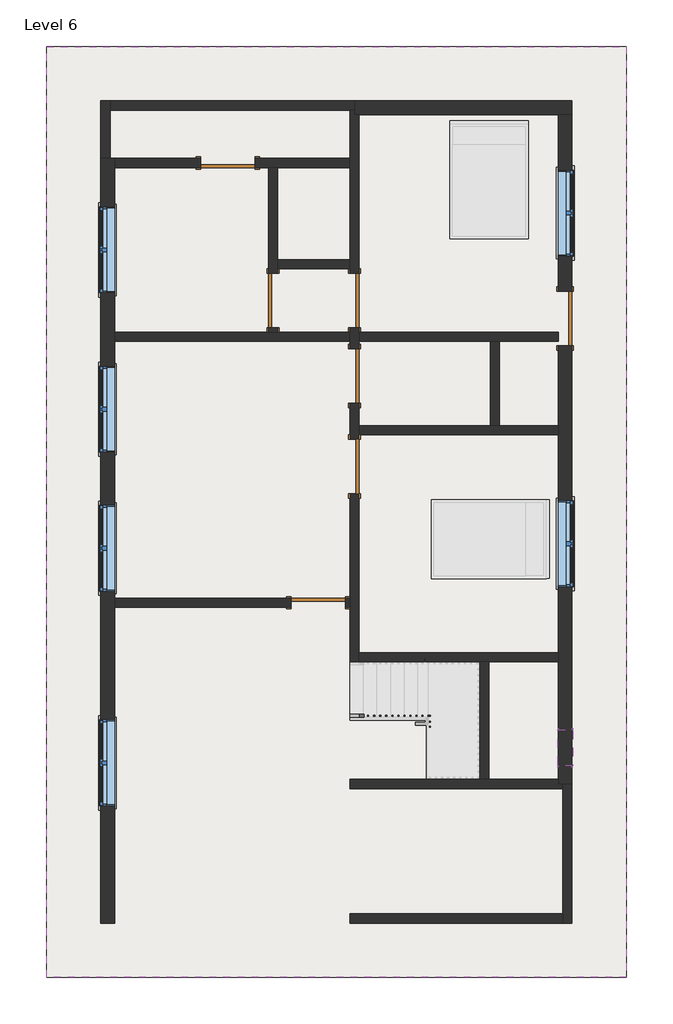
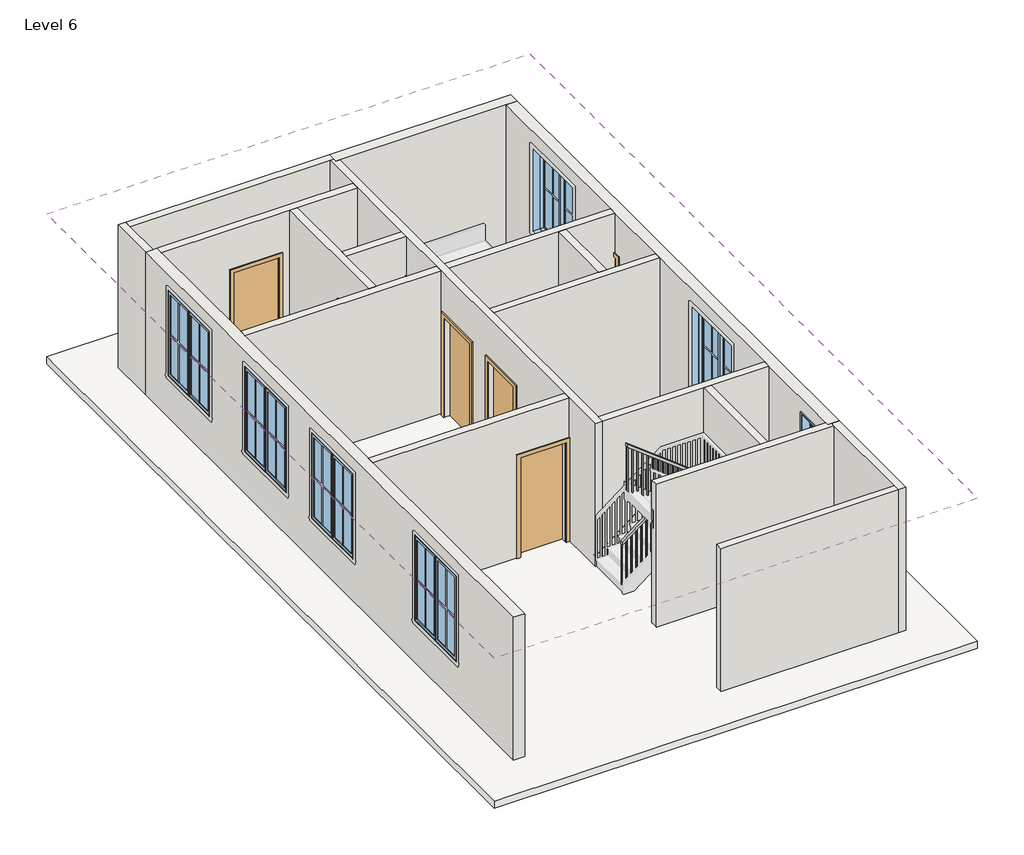
# One storey, part 1 of 2: 18 walls, 7 doors, 7 windows, 2 roofs, 1 railing.
"""IFC4 building model written with IfcOpenShell, lengths in millimetres."""

from ifc_helpers import new_model, si_unit, frame, origin, place, context, project, spatial, polyline, outline, extrude, faceted_brep, transform, mapped, element, save
from components import door_686f89d2, door_16372e1c, door_0ca8825f, window_9ac97e1a, window_f2d8fef0

model = new_model("IFC4")

# Units and contexts
model_context = context("Model", 3, world=origin())
ifc_project = project(units=[si_unit("LENGTHUNIT", "METRE", prefix="MILLI")], contexts=[model_context])

# Site, building, storey
site = spatial("IfcSite", under=ifc_project)
building = spatial("IfcBuilding", under=site)
storey = spatial("IfcBuildingStorey", under=building, Name="Level 6", Elevation=12801.6)

# Doors
placement = place(None, origin())
door_shape = door_686f89d2(model_context)
element("IfcDoor", 1, ObjectType="Single-Flush : 36\" x 84\"", at=placement, inside=storey, context=model_context, shape_type="MappedRepresentation", body=[
    mapped(door_shape, transform((-2318.0415352, 3143.9226491, 12801.6), x_axis=(0.0, -1.0, 0.0), y_axis=(1.0, 0.0, 0.0), z_axis=(0.0, 0.0, 1.0))),
])
element("IfcDoor", 2, ObjectType="Single-Flush : 36\" x 84\"", at=placement, inside=storey, context=model_context, shape_type="MappedRepresentation", body=[
    mapped(door_shape, transform((-946.4415352, 3143.7222669, 12801.6), x_axis=(0.0, 1.0, 0.0), y_axis=(-1.0, 0.0, 0.0), z_axis=(0.0, 0.0, 1.0))),
])
element("IfcDoor", 3, ObjectType="Single-Flush : 36\" x 84\"", at=placement, inside=storey, context=model_context, shape_type="MappedRepresentation", body=[
    mapped(door_shape, transform((-946.4415352, 1874.1230313, 12801.6), x_axis=(0.0, 1.0, 0.0), y_axis=(-1.0, 0.0, 0.0), z_axis=(0.0, 0.0, 1.0))),
])
element("IfcDoor", 4, ObjectType="Single-Flush : 36\" x 84\"", at=placement, inside=storey, context=model_context, shape_type="MappedRepresentation", body=[
    mapped(door_shape, transform((-946.4415352, 350.1230313, 12801.6), x_axis=(0.0, 1.0, 0.0), y_axis=(-1.0, 0.0, 0.0), z_axis=(0.0, 0.0, 1.0))),
])
element("IfcDoor", 5, ObjectType="Single-Flush : 36\" x 84\"", at=placement, inside=storey, context=model_context, shape_type="MappedRepresentation", body=[
    mapped(door_shape, transform((-3080.0415352, 5453.9645078, 12801.6), x_axis=(1.0, 0.0, 0.0), y_axis=(0.0, 1.0, 0.0), z_axis=(0.0, 0.0, 1.0))),
])
door_2_shape = door_16372e1c(model_context)
element("IfcDoor", 6, ObjectType="Single-Flush : 36\" x 84\"", at=placement, inside=storey, context=model_context, shape_type="MappedRepresentation", body=[
    mapped(door_2_shape, transform((-1556.0415352, -1935.8769687, 12801.6), x_axis=(1.0, 0.0, 0.0), y_axis=(0.0, 1.0, 0.0), z_axis=(0.0, 0.0, 1.0))),
])
door_3_shape = door_0ca8825f(model_context)
element("IfcDoor", 7, ObjectType="Single-Flush : 36\" x 84\"", at=placement, inside=storey, context=model_context, shape_type="MappedRepresentation", body=[
    mapped(door_3_shape, transform((2596.8584648, 2839.3230313, 12801.6), x_axis=(0.0, -1.0, 0.0), y_axis=(1.0, 0.0, 0.0), z_axis=(0.0, 0.0, 1.0))),
])

# Railing
element("IfcRailing", 8, ObjectType="Handrail - Rectangular", at=placement, inside=storey, context=model_context, shape_type="SolidModel", body=[
    faceted_brep([(-1022.6415352, -3810.4539367, 13885.3333333), (-1022.6415352, -3810.4539367, 13821.1783974), (-1022.6415352, -3861.2539367, 13821.1783974), (-1022.6415352, -3861.2539367, 13885.3333333), (218.4221038, -3810.4539367, 14842.5605883), (269.2221038, -3810.4539367, 14817.5874824), (269.2221038, -3861.2539367, 14817.5874824), (218.4221038, -3861.2539367, 14842.5605883), (218.4221038, -3810.4539367, 14901.3333333), (269.2221038, -3810.4539367, 14850.5333333), (269.2221038, -3861.2539367, 14850.5333333), (218.4221038, -3861.2539367, 14901.3333333), (345.4221038, -3810.4539367, 14901.3333333), (345.4221038, -3810.4539367, 14850.5333333), (294.6221038, -3861.2539367, 14850.5333333), (294.6221038, -3861.2539367, 14901.3333333), (345.4221038, -3937.4539367, 14901.3333333), (345.4221038, -3937.4539367, 14850.5333333), (294.6221038, -3937.4539367, 14850.5333333), (294.6221038, -3937.4539367, 14901.3333333), (345.4221038, -3993.2769687, 14901.3333333), (294.6221038, -3993.2769687, 14901.3333333), (294.6221038, -4044.0769687, 14850.5333333), (345.4221038, -4044.0769687, 14850.5333333)], [[[0, 1, 2, 3]], [[1, 0, 4, 5]], [[2, 1, 5, 6]], [[3, 2, 6, 7]], [[0, 3, 7, 4]], [[5, 4, 8, 9]], [[6, 5, 9, 10]], [[7, 6, 10, 11]], [[4, 7, 11, 8]], [[9, 8, 12, 13]], [[10, 9, 13, 14]], [[11, 10, 14, 15]], [[8, 11, 15, 12]], [[13, 12, 16, 17]], [[14, 13, 17, 18]], [[15, 14, 18, 19]], [[12, 15, 19, 16]], [[20, 21, 22, 23]], [[17, 16, 20, 23]], [[18, 17, 23, 22]], [[19, 18, 22, 21]], [[16, 19, 21, 20]]]),
    faceted_brep([(345.4221038, -3993.2769687, 14901.3333333), (345.4221038, -4044.0769687, 14850.5333333), (294.6221038, -4044.0769687, 14850.5333333), (294.6221038, -3993.2769687, 14901.3333333), (345.4221038, -3993.2769687, 15031.4848366), (294.6221038, -3993.2769687, 15006.5117307), (294.6221038, -4044.0769687, 15006.5117307), (345.4221038, -4044.0769687, 15031.4848366)], [[[0, 1, 2, 3]], [[4, 5, 6, 7]], [[1, 0, 4, 7]], [[2, 1, 7, 6]], [[3, 2, 6, 5]], [[0, 3, 5, 4]]]),
    faceted_brep([(345.4221038, -4044.0769687, 15031.4848366), (294.6221038, -4044.0769687, 15006.5117307), (294.6221038, -3993.2769687, 15006.5117307), (345.4221038, -3993.2769687, 15031.4848366), (-1022.6415352, -4044.0769687, 16086.6666667), (-1022.6415352, -3993.2769687, 16086.6666667), (-1022.6415352, -3993.2769687, 16022.5117307), (-1022.6415352, -4044.0769687, 16022.5117307)], [[[0, 1, 2, 3]], [[4, 5, 6, 7]], [[1, 0, 4, 7]], [[2, 1, 7, 6]], [[3, 2, 6, 5]], [[0, 3, 5, 4]]]),
    extrude(outline(polyline([(15998.3018032, -991.2528962), (16012.9949894, -1010.3028962), (15002.9333333, -1010.3028962), (15002.9333333, -991.2528962), (15998.3018032, -991.2528962)])), frame((0.0, -4028.2019687, 0.0), z_axis=(0.0, 1.0, 0.0), x_axis=(0.0, 0.0, 1.0)), (0.0, 0.0, 1.0), 19.05),
    extrude(outline(polyline([(15919.9381431, -889.6528962), (15934.6313294, -908.7028962), (15002.9333333, -908.7028962), (15002.9333333, -889.6528962), (15919.9381431, -889.6528962)])), frame((0.0, -4028.2019687, 0.0), z_axis=(0.0, 1.0, 0.0), x_axis=(0.0, 0.0, 1.0)), (0.0, 0.0, 1.0), 19.05),
    extrude(outline(polyline([(15841.5744831, -788.0528962), (15856.2676694, -807.1028962), (15002.9333333, -807.1028962), (15002.9333333, -788.0528962), (15841.5744831, -788.0528962)])), frame((0.0, -4028.2019687, 0.0), z_axis=(0.0, 1.0, 0.0), x_axis=(0.0, 0.0, 1.0)), (0.0, 0.0, 1.0), 19.05),
    extrude(outline(polyline([(15763.2108231, -686.4528962), (15777.9040093, -705.5028962), (14833.6, -705.5028962), (14833.6, -686.4528962), (15763.2108231, -686.4528962)])), frame((0.0, -4028.2019687, 0.0), z_axis=(0.0, 1.0, 0.0), x_axis=(0.0, 0.0, 1.0)), (0.0, 0.0, 1.0), 19.05),
    extrude(outline(polyline([(15684.847163, -584.8528962), (15699.5403493, -603.9028962), (14833.6, -603.9028962), (14833.6, -584.8528962), (15684.847163, -584.8528962)])), frame((0.0, -4028.2019687, 0.0), z_axis=(0.0, 1.0, 0.0), x_axis=(0.0, 0.0, 1.0)), (0.0, 0.0, 1.0), 19.05),
    extrude(outline(polyline([(15606.483503, -483.2528962), (15621.1766892, -502.3028962), (14664.2666667, -502.3028962), (14664.2666667, -483.2528962), (15606.483503, -483.2528962)])), frame((0.0, -4028.2019687, 0.0), z_axis=(0.0, 1.0, 0.0), x_axis=(0.0, 0.0, 1.0)), (0.0, 0.0, 1.0), 19.05),
    extrude(outline(polyline([(15528.1198429, -381.6528962), (15542.8130292, -400.7028962), (14664.2666667, -400.7028962), (14664.2666667, -381.6528962), (15528.1198429, -381.6528962)])), frame((0.0, -4028.2019687, 0.0), z_axis=(0.0, 1.0, 0.0), x_axis=(0.0, 0.0, 1.0)), (0.0, 0.0, 1.0), 19.05),
    extrude(outline(polyline([(15449.7561829, -280.0528962), (15464.4493691, -299.1028962), (14494.9333333, -299.1028962), (14494.9333333, -280.0528962), (15449.7561829, -280.0528962)])), frame((0.0, -4028.2019687, 0.0), z_axis=(0.0, 1.0, 0.0), x_axis=(0.0, 0.0, 1.0)), (0.0, 0.0, 1.0), 19.05),
    extrude(outline(polyline([(15371.3925228, -178.4528962), (15386.0857091, -197.5028962), (14494.9333333, -197.5028962), (14494.9333333, -178.4528962), (15371.3925228, -178.4528962)])), frame((0.0, -4028.2019687, 0.0), z_axis=(0.0, 1.0, 0.0), x_axis=(0.0, 0.0, 1.0)), (0.0, 0.0, 1.0), 19.05),
    extrude(outline(polyline([(15293.0288628, -76.8528962), (15307.722049, -95.9028962), (14325.6, -95.9028962), (14325.6, -76.8528962), (15293.0288628, -76.8528962)])), frame((0.0, -4028.2019687, 0.0), z_axis=(0.0, 1.0, 0.0), x_axis=(0.0, 0.0, 1.0)), (0.0, 0.0, 1.0), 19.05),
    extrude(outline(polyline([(15214.6652027, 24.7471038), (15229.358389, 5.6971038), (14325.6, 5.6971038), (14325.6, 24.7471038), (15214.6652027, 24.7471038)])), frame((0.0, -4028.2019687, 0.0), z_axis=(0.0, 1.0, 0.0), x_axis=(0.0, 0.0, 1.0)), (0.0, 0.0, 1.0), 19.05),
    extrude(outline(polyline([(15136.3015427, 126.3471038), (15150.9947289, 107.2971038), (14325.6, 107.2971038), (14325.6, 126.3471038), (15136.3015427, 126.3471038)])), frame((0.0, -4028.2019687, 0.0), z_axis=(0.0, 1.0, 0.0), x_axis=(0.0, 0.0, 1.0)), (0.0, 0.0, 1.0), 19.05),
    extrude(outline(polyline([(15057.9378826, 227.9471038), (15072.6310689, 208.8971038), (14156.2666667, 208.8971038), (14156.2666667, 227.9471038), (15057.9378826, 227.9471038)])), frame((0.0, -4028.2019687, 0.0), z_axis=(0.0, 1.0, 0.0), x_axis=(0.0, 0.0, 1.0)), (0.0, 0.0, 1.0), 19.05),
    extrude(outline(polyline([(310.4971038, -3927.9289367), (329.5471038, -3927.9289367), (329.5471038, -3946.9789367), (310.4971038, -3946.9789367), (310.4971038, -3927.9289367)])), frame((0.0, 0.0, 13986.9333333), z_axis=(0.0, 0.0, 1.0), x_axis=(1.0, 0.0, 0.0)), (0.0, 0.0, 1.0), 863.6),
    extrude(outline(polyline([(288.6334648, -3845.3789367), (288.6334648, -3826.3289367), (307.6834648, -3826.3289367), (307.6834648, -3845.3789367), (288.6334648, -3845.3789367)])), frame((0.0, 0.0, 13986.9333333), z_axis=(0.0, 0.0, 1.0), x_axis=(1.0, 0.0, 0.0)), (0.0, 0.0, 1.0), 863.6),
    extrude(outline(polyline([(14768.8889111, 206.0834648), (14754.1957248, 187.0334648), (13817.6, 187.0334648), (13817.6, 206.0834648), (14768.8889111, 206.0834648)])), frame((0.0, -3845.3789367, 0.0), z_axis=(0.0, 1.0, 0.0), x_axis=(0.0, 0.0, 1.0)), (0.0, 0.0, 1.0), 19.05),
    extrude(outline(polyline([(14690.525251, 104.4834648), (14675.8320648, 85.4334648), (13648.2666667, 85.4334648), (13648.2666667, 104.4834648), (14690.525251, 104.4834648)])), frame((0.0, -3845.3789367, 0.0), z_axis=(0.0, 1.0, 0.0), x_axis=(0.0, 0.0, 1.0)), (0.0, 0.0, 1.0), 19.05),
    extrude(outline(polyline([(14612.161591, 2.8834648), (14597.4684047, -16.1665352), (13648.2666667, -16.1665352), (13648.2666667, 2.8834648), (14612.161591, 2.8834648)])), frame((0.0, -3845.3789367, 0.0), z_axis=(0.0, 1.0, 0.0), x_axis=(0.0, 0.0, 1.0)), (0.0, 0.0, 1.0), 19.05),
    extrude(outline(polyline([(14533.7979309, -98.7165352), (14519.1047447, -117.7665352), (13648.2666667, -117.7665352), (13648.2666667, -98.7165352), (14533.7979309, -98.7165352)])), frame((0.0, -3845.3789367, 0.0), z_axis=(0.0, 1.0, 0.0), x_axis=(0.0, 0.0, 1.0)), (0.0, 0.0, 1.0), 19.05),
    extrude(outline(polyline([(14455.4342709, -200.3165352), (14440.7410846, -219.3665352), (13478.9333333, -219.3665352), (13478.9333333, -200.3165352), (14455.4342709, -200.3165352)])), frame((0.0, -3845.3789367, 0.0), z_axis=(0.0, 1.0, 0.0), x_axis=(0.0, 0.0, 1.0)), (0.0, 0.0, 1.0), 19.05),
    extrude(outline(polyline([(14377.0706109, -301.9165352), (14362.3774246, -320.9665352), (13478.9333333, -320.9665352), (13478.9333333, -301.9165352), (14377.0706109, -301.9165352)])), frame((0.0, -3845.3789367, 0.0), z_axis=(0.0, 1.0, 0.0), x_axis=(0.0, 0.0, 1.0)), (0.0, 0.0, 1.0), 19.05),
    extrude(outline(polyline([(14298.7069508, -403.5165352), (14284.0137645, -422.5665352), (13309.6, -422.5665352), (13309.6, -403.5165352), (14298.7069508, -403.5165352)])), frame((0.0, -3845.3789367, 0.0), z_axis=(0.0, 1.0, 0.0), x_axis=(0.0, 0.0, 1.0)), (0.0, 0.0, 1.0), 19.05),
    extrude(outline(polyline([(14220.3432908, -505.1165352), (14205.6501045, -524.1665352), (13309.6, -524.1665352), (13309.6, -505.1165352), (14220.3432908, -505.1165352)])), frame((0.0, -3845.3789367, 0.0), z_axis=(0.0, 1.0, 0.0), x_axis=(0.0, 0.0, 1.0)), (0.0, 0.0, 1.0), 19.05),
    extrude(outline(polyline([(14141.9796307, -606.7165352), (14127.2864445, -625.7665352), (13140.2666667, -625.7665352), (13140.2666667, -606.7165352), (14141.9796307, -606.7165352)])), frame((0.0, -3845.3789367, 0.0), z_axis=(0.0, 1.0, 0.0), x_axis=(0.0, 0.0, 1.0)), (0.0, 0.0, 1.0), 19.05),
    extrude(outline(polyline([(14063.6159707, -708.3165352), (14048.9227844, -727.3665352), (13140.2666667, -727.3665352), (13140.2666667, -708.3165352), (14063.6159707, -708.3165352)])), frame((0.0, -3845.3789367, 0.0), z_axis=(0.0, 1.0, 0.0), x_axis=(0.0, 0.0, 1.0)), (0.0, 0.0, 1.0), 19.05),
    extrude(outline(polyline([(13985.2523106, -809.9165352), (13970.5591244, -828.9665352), (12970.9333333, -828.9665352), (12970.9333333, -809.9165352), (13985.2523106, -809.9165352)])), frame((0.0, -3845.3789367, 0.0), z_axis=(0.0, 1.0, 0.0), x_axis=(0.0, 0.0, 1.0)), (0.0, 0.0, 1.0), 19.05),
    extrude(outline(polyline([(13906.8886506, -911.5165352), (13892.1954643, -930.5665352), (12970.9333333, -930.5665352), (12970.9333333, -911.5165352), (13906.8886506, -911.5165352)])), frame((0.0, -3845.3789367, 0.0), z_axis=(0.0, 1.0, 0.0), x_axis=(0.0, 0.0, 1.0)), (0.0, 0.0, 1.0), 19.05),
    extrude(outline(polyline([(310.4971038, -4009.1519687), (329.5471038, -4009.1519687), (329.5471038, -4028.2019687), (310.4971038, -4028.2019687), (310.4971038, -4009.1519687)])), frame((0.0, 0.0, 13986.9333333), z_axis=(0.0, 0.0, 1.0), x_axis=(1.0, 0.0, 0.0)), (0.0, 0.0, 1.0), 863.6),
    extrude(outline(polyline([(310.4971038, -3845.3789367), (310.4971038, -3826.3289367), (329.5471038, -3826.3289367), (329.5471038, -3845.3789367), (310.4971038, -3845.3789367)])), frame((0.0, 0.0, 13986.9333333), z_axis=(0.0, 0.0, 1.0), x_axis=(1.0, 0.0, 0.0)), (0.0, 0.0, 1.0), 863.6),
    extrude(outline(polyline([(16007.8185445, -1003.5915352), (16022.5117307, -1022.6415352), (15002.9333333, -1022.6415352), (15002.9333333, -1003.5915352), (16007.8185445, -1003.5915352)])), frame((0.0, -4028.2019687, 0.0), z_axis=(0.0, 1.0, 0.0), x_axis=(0.0, 0.0, 1.0)), (0.0, 0.0, 1.0), 19.05),
    extrude(outline(polyline([(13835.8715837, -1003.5915352), (13821.1783974, -1022.6415352), (12970.9333333, -1022.6415352), (12970.9333333, -1003.5915352), (13835.8715837, -1003.5915352)])), frame((0.0, -3845.3789367, 0.0), z_axis=(0.0, 1.0, 0.0), x_axis=(0.0, 0.0, 1.0)), (0.0, 0.0, 1.0), 19.05),
])

# Roofs
element("IfcRoof", 9, ObjectType="ROOF 6\"", at=placement, inside=storey, context=model_context, shape_type="SweptSolid", body=[
    extrude(outline(polyline([(-6128.0415352, 7411.3230313), (3625.5584648, 7411.3230313), (3625.5584648, -8235.0769687), (-6128.0415352, -8235.0769687), (-6128.0415352, 7411.3230313)])), frame((0.0, 0.0, 12649.2), z_axis=(0.0, 0.0, 1.0), x_axis=(1.0, 0.0, 0.0)), (0.0, 0.0, 1.0), 152.4),
])
element("IfcRoof", 10, ObjectType="ROOF 6\"", at=placement, inside=storey, context=model_context, shape_type="SweptSolid", body=[
    extrude(outline(polyline([(-6128.0415352, 7411.3230313), (3625.5584648, 7411.3230313), (3625.5584648, -8235.0769687), (-6128.0415352, -8235.0769687), (-6128.0415352, 7411.3230313)])), frame((0.0, 0.0, 15849.6), z_axis=(0.0, 0.0, 1.0), x_axis=(1.0, 0.0, 0.0)), (0.0, 0.0, 1.0), 152.4),
])

# Walls
element("IfcWall", 11, ObjectType="WALL 6\"", at=placement, inside=storey, context=model_context, shape_type="Brep", body=[
    faceted_brep([(-5061.2415352, 5531.7230313, 12801.6), (-5061.2415352, 6344.5230313, 12801.6), (-5061.2415352, 6496.9230313, 12801.6), (-5061.2415352, 6496.9230313, 15849.6), (-5061.2415352, 6344.5230313, 15849.6), (-5061.2415352, 5531.7230313, 15849.6), (-5213.6415352, 5531.7230313, 12801.6), (-5213.6415352, 5531.7230313, 15849.6), (-5213.6415352, 6496.9230313, 15849.6), (-5213.6415352, 6496.9230313, 12801.6)], [[[0, 1, 2, 3, 4, 5]], [[6, 7, 8, 9]], [[2, 1, 0, 6, 9]], [[0, 5, 7, 6]], [[3, 2, 9, 8]], [[5, 4, 3, 8, 7]]]),
])
element("IfcWall", 12, ObjectType="WALL 6\"", at=placement, inside=storey, context=model_context, shape_type="Brep", body=[
    faceted_brep([(-5061.2415352, 6344.5230313, 12801.6), (-1022.6415352, 6344.5230313, 12801.6), (-946.4415352, 6344.5230313, 12801.6), (-946.4415352, 6344.5230313, 15849.6), (-1022.6415352, 6344.5230313, 15849.6), (-5061.2415352, 6344.5230313, 15849.6), (-5061.2415352, 6496.9230313, 12801.6), (-5061.2415352, 6496.9230313, 15849.6), (-946.4415352, 6496.9230313, 15849.6), (-946.4415352, 6496.9230313, 12801.6)], [[[0, 1, 2, 3, 4, 5]], [[6, 7, 8, 9]], [[2, 1, 0, 6, 9]], [[3, 2, 9, 8]], [[0, 5, 7, 6]], [[5, 4, 3, 8, 7]]]),
])
element("IfcWall", 13, ObjectType="WALL 6\"", at=placement, inside=storey, context=model_context, shape_type="Brep", body=[
    faceted_brep([(-1022.6415352, 1416.9230313, 12801.6), (-1022.6415352, 807.3230313, 12801.6), (-1022.6415352, 807.3230313, 14935.2), (-1022.6415352, -107.0769687, 14935.2), (-1022.6415352, -107.0769687, 12801.6), (-1022.6415352, -1859.6769687, 12801.6), (-1022.6415352, -2012.0769687, 12801.6), (-1022.6415352, -2926.4769687, 12801.6), (-1022.6415352, -2926.4769687, 15849.6), (-1022.6415352, -2012.0769687, 15849.6), (-1022.6415352, -1859.6769687, 15849.6), (-1022.6415352, 2458.3230313, 15849.6), (-1022.6415352, 2610.7230313, 15849.6), (-1022.6415352, 3677.1222669, 15849.6), (-1022.6415352, 3829.5222669, 15849.6), (-1022.6415352, 5377.7645078, 15849.6), (-1022.6415352, 5530.1645078, 15849.6), (-1022.6415352, 6344.5230313, 15849.6), (-1022.6415352, 6344.5230313, 12801.6), (-1022.6415352, 5530.1645078, 12801.6), (-1022.6415352, 5377.7645078, 12801.6), (-1022.6415352, 3829.5222669, 12801.6), (-1022.6415352, 3677.1222669, 12801.6), (-1022.6415352, 3600.9222669, 12801.6), (-1022.6415352, 3600.9222669, 14935.2), (-1022.6415352, 2686.5222669, 14935.2), (-1022.6415352, 2686.5222669, 12801.6), (-1022.6415352, 2610.7230313, 12801.6), (-1022.6415352, 2458.3230313, 12801.6), (-1022.6415352, 2331.3230313, 12801.6), (-1022.6415352, 2331.3230313, 14935.2), (-1022.6415352, 1416.9230313, 14935.2), (-870.2415352, 807.3230313, 14935.2), (-870.2415352, 807.3230313, 12801.6), (-870.2415352, 883.5230313, 12801.6), (-870.2415352, 1035.9230313, 12801.6), (-870.2415352, 1416.9230313, 12801.6), (-870.2415352, 1416.9230313, 14935.2), (-870.2415352, 2331.3230313, 14935.2), (-870.2415352, 2331.3230313, 12801.6), (-870.2415352, 2458.3230313, 12801.6), (-870.2415352, 2610.7230313, 12801.6), (-870.2415352, 2686.5222669, 12801.6), (-870.2415352, 2686.5222669, 14935.2), (-870.2415352, 3600.9222669, 14935.2), (-870.2415352, 3600.9222669, 12801.6), (-870.2415352, 6268.3230313, 12801.6), (-870.2415352, 6268.3230313, 15849.6), (-870.2415352, 2610.7230313, 15849.6), (-870.2415352, 2458.3230313, 15849.6), (-870.2415352, 1035.9230313, 15849.6), (-870.2415352, 883.5230313, 15849.6), (-870.2415352, -2774.0769687, 15849.6), (-870.2415352, -2926.4769687, 15849.6), (-870.2415352, -2926.4769687, 12801.6), (-870.2415352, -2774.0769687, 12801.6), (-870.2415352, -107.0769687, 12801.6), (-870.2415352, -107.0769687, 14935.2), (-946.4415352, 6344.5230313, 12801.6), (-946.4415352, 6268.3230313, 12801.6), (-946.4415352, 6344.5230313, 15849.6), (-946.4415352, 6268.3230313, 15849.6)], [[[0, 1, 2, 3, 4, 5, 6, 7, 8, 9, 10, 11, 12, 13, 14, 15, 16, 17, 18, 19, 20, 21, 22, 23, 24, 25, 26, 27, 28, 29, 30, 31]], [[32, 33, 34, 35, 36, 37, 38, 39, 40, 41, 42, 43, 44, 45, 46, 47, 48, 49, 50, 51, 52, 53, 54, 55, 56, 57]], [[46, 45, 23, 22, 21, 20, 19, 18, 58, 59]], [[42, 41, 40, 39, 29, 28, 27, 26]], [[56, 55, 54, 7, 6, 5, 4]], [[36, 35, 34, 33, 1, 0]], [[18, 17, 60, 58]], [[60, 61, 59, 58]], [[61, 47, 46, 59]], [[8, 7, 54, 53]], [[24, 23, 45, 44]], [[25, 24, 44, 43]], [[26, 25, 43, 42]], [[30, 29, 39, 38]], [[31, 30, 38, 37]], [[0, 31, 37, 36]], [[2, 1, 33, 32]], [[3, 2, 32, 57]], [[4, 3, 57, 56]], [[17, 16, 15, 14, 13, 12, 11, 10, 9, 8, 53, 52, 51, 50, 49, 48, 47, 61, 60]]]),
])
element("IfcWall", 14, ObjectType="WALL 6\"", at=placement, inside=storey, context=model_context, shape_type="Brep", body=[
    faceted_brep([(2482.5584648, -2774.0769687, 12801.6), (-870.2415352, -2774.0769687, 12801.6), (-870.2415352, -2774.0769687, 15849.6), (2482.5584648, -2774.0769687, 15849.6), (2482.5584648, -2926.4769687, 12801.6), (2482.5584648, -2926.4769687, 15849.6), (1314.1584648, -2926.4769687, 15849.6), (1161.7584648, -2926.4769687, 15849.6), (-870.2415352, -2926.4769687, 15849.6), (-870.2415352, -2926.4769687, 12801.6), (1161.7584648, -2926.4769687, 12801.6), (1314.1584648, -2926.4769687, 12801.6)], [[[0, 1, 2, 3]], [[4, 5, 6, 7, 8, 9, 10, 11]], [[1, 0, 4, 11, 10, 9]], [[2, 1, 9, 8]], [[0, 3, 5, 4]], [[3, 2, 8, 7, 6, 5]]]),
])
element("IfcWall", 15, ObjectType="WALL 6\"", at=placement, inside=storey, context=model_context, shape_type="Brep", body=[
    faceted_brep([(2558.7584648, -4983.8769687, 12801.6), (2558.7584648, -5060.0769687, 12801.6), (2558.7584648, -7168.2769687, 12801.6), (2558.7584648, -7320.6769687, 12801.6), (2558.7584648, -7320.6769687, 15849.6), (2558.7584648, -7168.2769687, 15849.6), (2558.7584648, -5060.0769687, 15849.6), (2558.7584648, -4983.8769687, 15849.6), (2711.1584648, -4983.8769687, 12801.6), (2711.1584648, -4983.8769687, 15849.6), (2711.1584648, -7320.6769687, 15849.6), (2711.1584648, -7320.6769687, 12801.6)], [[[0, 1, 2, 3, 4, 5, 6, 7]], [[8, 9, 10, 11]], [[3, 2, 1, 0, 8, 11]], [[0, 7, 9, 8]], [[4, 3, 11, 10]], [[7, 6, 5, 4, 10, 9]]]),
])
element("IfcWall", 16, ObjectType="WALL 6\"", at=placement, inside=storey, context=model_context, shape_type="SweptSolid", body=[
    extrude(outline(polyline([(-1022.6415352, -7168.2769687), (2558.7584648, -7168.2769687), (2558.7584648, -7320.6769687), (-1022.6415352, -7320.6769687), (-1022.6415352, -7168.2769687)])), frame((0.0, 0.0, 12801.6), z_axis=(0.0, 0.0, 1.0), x_axis=(1.0, 0.0, 0.0)), (0.0, 0.0, 1.0), 3048.0),
])
element("IfcWall", 17, ObjectType="WALL 6\"", at=placement, inside=storey, context=model_context, shape_type="Brep", body=[
    faceted_brep([(2482.5584648, -4907.6769687, 12801.6), (1314.1584648, -4907.6769687, 12801.6), (1161.7584648, -4907.6769687, 12801.6), (-1022.6415352, -4907.6769687, 12801.6), (-1022.6415352, -4907.6769687, 15849.6), (1161.7584648, -4907.6769687, 15849.6), (1314.1584648, -4907.6769687, 15849.6), (2482.5584648, -4907.6769687, 15849.6), (2558.7584648, -5060.0769687, 12801.6), (2558.7584648, -5060.0769687, 15849.6), (-1022.6415352, -5060.0769687, 15849.6), (-1022.6415352, -5060.0769687, 12801.6), (2482.5584648, -4983.8769687, 12801.6), (2558.7584648, -4983.8769687, 12801.6), (2482.5584648, -4983.8769687, 15849.6), (2558.7584648, -4983.8769687, 15849.6)], [[[0, 1, 2, 3, 4, 5, 6, 7]], [[8, 9, 10, 11]], [[3, 2, 1, 0, 12, 13, 8, 11]], [[4, 3, 11, 10]], [[0, 7, 14, 12]], [[14, 15, 13, 12]], [[15, 9, 8, 13]], [[7, 6, 5, 4, 10, 9, 15, 14]]]),
])
element("IfcWall", 18, ObjectType="WALL 6\"", at=placement, inside=storey, context=model_context, shape_type="SweptSolid", body=[
    extrude(outline(polyline([(1161.7584648, -4907.6769687), (1161.7584648, -2926.4769687), (1314.1584648, -2926.4769687), (1314.1584648, -4907.6769687), (1161.7584648, -4907.6769687)])), frame((0.0, 0.0, 12801.6), z_axis=(0.0, 0.0, 1.0), x_axis=(1.0, 0.0, 0.0)), (0.0, 0.0, 1.0), 3048.0),
])
element("IfcWall", 19, ObjectType="WALL 6\"", at=placement, inside=storey, context=model_context, shape_type="SweptSolid", body=[
    extrude(outline(polyline([(14935.2, -1098.8415352), (12801.6, -1098.8415352), (12801.6, -1022.6415352), (15849.6, -1022.6415352), (15849.6, -4985.0415352), (12801.6, -4985.0415352), (12801.6, -2013.2415352), (14935.2, -2013.2415352), (14935.2, -1098.8415352)])), frame((0.0, -2012.0769687, 0.0), z_axis=(0.0, 1.0, 0.0), x_axis=(0.0, 0.0, 1.0)), (0.0, 0.0, 1.0), 152.4),
])
element("IfcWall", 20, ObjectType="WALL 6\"", at=placement, inside=storey, context=model_context, shape_type="Brep", body=[
    faceted_brep([(2482.5584648, 2458.3230313, 12801.6), (2482.5584648, 2458.3230313, 15849.6), (1491.9584648, 2458.3230313, 15849.6), (1339.5584648, 2458.3230313, 15849.6), (-870.2415352, 2458.3230313, 15849.6), (-870.2415352, 2458.3230313, 12801.6), (1339.5584648, 2458.3230313, 12801.6), (1491.9584648, 2458.3230313, 12801.6), (2482.5584648, 2610.7230313, 15849.6), (2482.5584648, 2610.7230313, 12801.6), (-870.2415352, 2610.7230313, 12801.6), (-870.2415352, 2610.7230313, 15849.6)], [[[0, 1, 2, 3, 4, 5, 6, 7]], [[8, 9, 10, 11]], [[9, 0, 7, 6, 5, 10]], [[1, 0, 9, 8]], [[5, 4, 11, 10]], [[1, 8, 11, 4, 3, 2]]]),
    faceted_brep([(-4985.0415352, 2458.3230313, 15849.6), (-4985.0415352, 2458.3230313, 12801.6), (-1022.6415352, 2458.3230313, 12801.6), (-1022.6415352, 2458.3230313, 15849.6), (-4985.0415352, 2610.7230313, 12801.6), (-4985.0415352, 2610.7230313, 15849.6), (-2394.2415352, 2610.7230313, 15849.6), (-2241.8415352, 2610.7230313, 15849.6), (-1022.6415352, 2610.7230313, 15849.6), (-1022.6415352, 2610.7230313, 12801.6), (-2241.8415352, 2610.7230313, 12801.6), (-2394.2415352, 2610.7230313, 12801.6)], [[[0, 1, 2, 3]], [[4, 5, 6, 7, 8, 9, 10, 11]], [[1, 4, 11, 10, 9, 2]], [[1, 0, 5, 4]], [[3, 2, 9, 8]], [[5, 0, 3, 8, 7, 6]]]),
])
element("IfcWall", 21, ObjectType="WALL 6\"", at=placement, inside=storey, context=model_context, shape_type="Brep", body=[
    faceted_brep([(-2622.8415352, 5377.7645078, 14935.2), (-2622.8415352, 5377.7645078, 12801.6), (-2394.2415352, 5377.7645078, 12801.6), (-2241.8415352, 5377.7645078, 12801.6), (-1022.6415352, 5377.7645078, 12801.6), (-1022.6415352, 5377.7645078, 15849.6), (-2241.8415352, 5377.7645078, 15849.6), (-2394.2415352, 5377.7645078, 15849.6), (-4985.0415352, 5377.7645078, 15849.6), (-4985.0415352, 5377.7645078, 12801.6), (-3537.2415352, 5377.7645078, 12801.6), (-3537.2415352, 5377.7645078, 14935.2), (-1022.6415352, 5530.1645078, 12801.6), (-2622.8415352, 5530.1645078, 12801.6), (-2622.8415352, 5530.1645078, 14935.2), (-3537.2415352, 5530.1645078, 14935.2), (-3537.2415352, 5530.1645078, 12801.6), (-4985.0415352, 5530.1645078, 12801.6), (-4985.0415352, 5530.1645078, 15849.6), (-1022.6415352, 5530.1645078, 15849.6)], [[[0, 1, 2, 3, 4, 5, 6, 7, 8, 9, 10, 11]], [[12, 13, 14, 15, 16, 17, 18, 19]], [[10, 9, 17, 16]], [[4, 3, 2, 1, 13, 12]], [[9, 8, 18, 17]], [[5, 4, 12, 19]], [[14, 13, 1, 0]], [[15, 14, 0, 11]], [[16, 15, 11, 10]], [[8, 7, 6, 5, 19, 18]]]),
])
element("IfcWall", 22, ObjectType="WALL 6\"", at=placement, inside=storey, context=model_context, shape_type="Brep", body=[
    faceted_brep([(-2394.2415352, 2686.7226491, 14935.2), (-2394.2415352, 2686.7226491, 12801.6), (-2394.2415352, 2610.7230313, 12801.6), (-2394.2415352, 2610.7230313, 15849.6), (-2394.2415352, 5377.7645078, 15849.6), (-2394.2415352, 5377.7645078, 12801.6), (-2394.2415352, 3601.1226491, 12801.6), (-2394.2415352, 3601.1226491, 14935.2), (-2241.8415352, 2610.7230313, 12801.6), (-2241.8415352, 2686.7226491, 12801.6), (-2241.8415352, 2686.7226491, 14935.2), (-2241.8415352, 3601.1226491, 14935.2), (-2241.8415352, 3601.1226491, 12801.6), (-2241.8415352, 3677.1222669, 12801.6), (-2241.8415352, 3829.5222669, 12801.6), (-2241.8415352, 5377.7645078, 12801.6), (-2241.8415352, 5377.7645078, 15849.6), (-2241.8415352, 3829.5222669, 15849.6), (-2241.8415352, 3677.1222669, 15849.6), (-2241.8415352, 2610.7230313, 15849.6)], [[[0, 1, 2, 3, 4, 5, 6, 7]], [[8, 9, 10, 11, 12, 13, 14, 15, 16, 17, 18, 19]], [[6, 5, 15, 14, 13, 12]], [[2, 1, 9, 8]], [[3, 2, 8, 19]], [[5, 4, 16, 15]], [[10, 9, 1, 0]], [[11, 10, 0, 7]], [[12, 11, 7, 6]], [[4, 3, 19, 18, 17, 16]]]),
])
element("IfcWall", 23, ObjectType="WALL 6\"", at=placement, inside=storey, context=model_context, shape_type="SweptSolid", body=[
    extrude(outline(polyline([(-1022.6415352, 3677.1222669), (-2241.8415352, 3677.1222669), (-2241.8415352, 3829.5222669), (-1022.6415352, 3829.5222669), (-1022.6415352, 3677.1222669)])), frame((0.0, 0.0, 12801.6), z_axis=(0.0, 0.0, 1.0), x_axis=(1.0, 0.0, 0.0)), (0.0, 0.0, 1.0), 3048.0),
])
element("IfcWall", 24, ObjectType="WALL 6\"", at=placement, inside=storey, context=model_context, shape_type="Brep", body=[
    faceted_brep([(-870.2415352, 883.5230313, 12801.6), (2482.5584648, 883.5230313, 12801.6), (2482.5584648, 883.5230313, 15849.6), (-870.2415352, 883.5230313, 15849.6), (-870.2415352, 1035.9230313, 12801.6), (-870.2415352, 1035.9230313, 15849.6), (1339.5584648, 1035.9230313, 15849.6), (1491.9584648, 1035.9230313, 15849.6), (2482.5584648, 1035.9230313, 15849.6), (2482.5584648, 1035.9230313, 12801.6), (1491.9584648, 1035.9230313, 12801.6), (1339.5584648, 1035.9230313, 12801.6)], [[[0, 1, 2, 3]], [[4, 5, 6, 7, 8, 9, 10, 11]], [[1, 0, 4, 11, 10, 9]], [[2, 1, 9, 8]], [[0, 3, 5, 4]], [[3, 2, 8, 7, 6, 5]]]),
])
element("IfcWall", 25, ObjectType="WALL 6\"", at=placement, inside=storey, context=model_context, shape_type="SweptSolid", body=[
    extrude(outline(polyline([(1339.5584648, 1035.9230313), (1339.5584648, 2458.3230313), (1491.9584648, 2458.3230313), (1491.9584648, 1035.9230313), (1339.5584648, 1035.9230313)])), frame((0.0, 0.0, 12801.6), z_axis=(0.0, 0.0, 1.0), x_axis=(1.0, 0.0, 0.0)), (0.0, 0.0, 1.0), 3048.0),
])
element("IfcWall", 26, ObjectType="WALL 9\"", at=placement, inside=storey, context=model_context, shape_type="Brep", body=[
    faceted_brep([(-946.4415352, 6268.3230313, 12801.6), (-870.2415352, 6268.3230313, 12801.6), (2482.5584648, 6268.3230313, 12801.6), (2711.1584648, 6268.3230313, 12801.6), (2711.1584648, 6268.3230313, 15849.6), (2482.5584648, 6268.3230313, 15849.6), (-870.2415352, 6268.3230313, 15849.6), (-946.4415352, 6268.3230313, 15849.6), (-946.4415352, 6496.9230313, 12801.6), (-946.4415352, 6496.9230313, 15849.6), (2711.1584648, 6496.9230313, 15849.6), (2711.1584648, 6496.9230313, 12801.6), (-946.4415352, 6344.5230313, 12801.6), (-946.4415352, 6344.5230313, 15849.6)], [[[0, 1, 2, 3, 4, 5, 6, 7]], [[8, 9, 10, 11]], [[3, 2, 1, 0, 12, 8, 11]], [[0, 7, 13, 9, 8, 12]], [[4, 3, 11, 10]], [[7, 6, 5, 4, 10, 9, 13]]]),
])
element("IfcWall", 27, ObjectType="WALL 9\"", at=placement, inside=storey, context=model_context, shape_type="Brep", body=[
    faceted_brep([(2482.5584648, 2382.1230313, 14935.2), (2482.5584648, 2382.1230313, 12801.6), (2482.5584648, 1035.9230313, 12801.6), (2482.5584648, 883.5230313, 12801.6), (2482.5584648, -2774.0769687, 12801.6), (2482.5584648, -2926.4769687, 12801.6), (2482.5584648, -4907.6769687, 12801.6), (2482.5584648, -4983.8769687, 12801.6), (2482.5584648, -4983.8769687, 15849.6), (2482.5584648, -4907.6769687, 15849.6), (2482.5584648, -2926.4769687, 15849.6), (2482.5584648, -2774.0769687, 15849.6), (2482.5584648, 883.5230313, 15849.6), (2482.5584648, 1035.9230313, 15849.6), (2482.5584648, 2458.3230313, 15849.6), (2482.5584648, 2610.7230313, 15849.6), (2482.5584648, 6268.3230313, 15849.6), (2482.5584648, 6268.3230313, 12801.6), (2482.5584648, 3296.5230313, 12801.6), (2482.5584648, 3296.5230313, 14935.2), (2482.5584648, 3887.0730313, 15544.8), (2482.5584648, 3887.0730313, 13716.0), (2482.5584648, 5334.8730313, 13716.0), (2482.5584648, 5334.8730313, 15544.8), (2482.5584648, -1669.1769687, 15544.8), (2482.5584648, -1669.1769687, 13716.0), (2482.5584648, -221.3769687, 13716.0), (2482.5584648, -221.3769687, 15544.8), (2482.5584648, -4069.4769687, 15544.8), (2482.5584648, -4679.0769687, 15544.8), (2482.5584648, -4679.0769687, 14935.2), (2482.5584648, -4069.4769687, 14935.2), (2711.1584648, -4983.8769687, 12801.6), (2711.1584648, 2382.1230313, 12801.6), (2711.1584648, 2382.1230313, 14935.2), (2711.1584648, 3296.5230313, 14935.2), (2711.1584648, 3296.5230313, 12801.6), (2711.1584648, 6268.3230313, 12801.6), (2711.1584648, 6268.3230313, 15849.6), (2711.1584648, -4983.8769687, 15849.6), (2711.1584648, 3887.0730313, 15544.8), (2711.1584648, 5334.8730313, 15544.8), (2711.1584648, 5334.8730313, 13716.0), (2711.1584648, 3887.0730313, 13716.0), (2711.1584648, -1669.1769687, 15544.8), (2711.1584648, -221.3769687, 15544.8), (2711.1584648, -221.3769687, 13716.0), (2711.1584648, -1669.1769687, 13716.0), (2711.1584648, -4069.4769687, 15544.8), (2711.1584648, -4069.4769687, 14935.2), (2711.1584648, -4679.0769687, 14935.2), (2711.1584648, -4679.0769687, 15544.8), (2558.7584648, -4983.8769687, 12801.6), (2558.7584648, -4983.8769687, 15849.6)], [[[0, 1, 2, 3, 4, 5, 6, 7, 8, 9, 10, 11, 12, 13, 14, 15, 16, 17, 18, 19], [20, 21, 22, 23], [24, 25, 26, 27], [28, 29, 30, 31]], [[32, 33, 34, 35, 36, 37, 38, 39], [40, 41, 42, 43], [44, 45, 46, 47], [48, 49, 50, 51]], [[18, 17, 37, 36]], [[7, 6, 5, 4, 3, 2, 1, 33, 32, 52]], [[8, 7, 52, 32, 39, 53]], [[17, 16, 38, 37]], [[34, 33, 1, 0]], [[35, 34, 0, 19]], [[36, 35, 19, 18]], [[21, 20, 40, 43]], [[22, 21, 43, 42]], [[23, 22, 42, 41]], [[20, 23, 41, 40]], [[25, 24, 44, 47]], [[26, 25, 47, 46]], [[27, 26, 46, 45]], [[24, 27, 45, 44]], [[49, 48, 28, 31]], [[50, 49, 31, 30]], [[51, 50, 30, 29]], [[48, 51, 29, 28]], [[16, 15, 14, 13, 12, 11, 10, 9, 8, 53, 39, 38]]]),
])
element("IfcWall", 28, ObjectType="WALL 9\"", at=placement, inside=storey, context=model_context, shape_type="Brep", body=[
    faceted_brep([(-4985.0415352, -7320.6769687, 12801.6), (-4985.0415352, -2012.0769687, 12801.6), (-4985.0415352, -1859.6769687, 12801.6), (-4985.0415352, 2458.3230313, 12801.6), (-4985.0415352, 2610.7230313, 12801.6), (-4985.0415352, 5377.7645078, 12801.6), (-4985.0415352, 5530.1645078, 12801.6), (-4985.0415352, 5531.7230313, 12801.6), (-4985.0415352, 5531.7230313, 15849.6), (-4985.0415352, 5530.1645078, 15849.6), (-4985.0415352, 5377.7645078, 15849.6), (-4985.0415352, 2610.7230313, 15849.6), (-4985.0415352, 2458.3230313, 15849.6), (-4985.0415352, -1859.6769687, 15849.6), (-4985.0415352, -2012.0769687, 15849.6), (-4985.0415352, -7320.6769687, 15849.6), (-4985.0415352, 4718.1437696, 15544.8), (-4985.0415352, 4718.1437696, 13716.0), (-4985.0415352, 3270.3437696, 13716.0), (-4985.0415352, 3270.3437696, 15544.8), (-4985.0415352, 2039.2230313, 15544.8), (-4985.0415352, 2039.2230313, 13716.0), (-4985.0415352, 591.4230313, 13716.0), (-4985.0415352, 591.4230313, 15544.8), (-4985.0415352, -297.5769687, 15544.8), (-4985.0415352, -297.5769687, 13716.0), (-4985.0415352, -1745.3769687, 13716.0), (-4985.0415352, -1745.3769687, 15544.8), (-4985.0415352, -3904.3769687, 15544.8), (-4985.0415352, -3904.3769687, 13716.0), (-4985.0415352, -5352.1769687, 13716.0), (-4985.0415352, -5352.1769687, 15544.8), (-5213.6415352, -7320.6769687, 12801.6), (-5213.6415352, -7320.6769687, 15849.6), (-5213.6415352, 5531.7230313, 15849.6), (-5213.6415352, 5531.7230313, 12801.6), (-5213.6415352, 4718.1437696, 15544.8), (-5213.6415352, 3270.3437696, 15544.8), (-5213.6415352, 3270.3437696, 13716.0), (-5213.6415352, 4718.1437696, 13716.0), (-5213.6415352, 2039.2230313, 15544.8), (-5213.6415352, 591.4230313, 15544.8), (-5213.6415352, 591.4230313, 13716.0), (-5213.6415352, 2039.2230313, 13716.0), (-5213.6415352, -297.5769687, 15544.8), (-5213.6415352, -1745.3769687, 15544.8), (-5213.6415352, -1745.3769687, 13716.0), (-5213.6415352, -297.5769687, 13716.0), (-5213.6415352, -3904.3769687, 15544.8), (-5213.6415352, -5352.1769687, 15544.8), (-5213.6415352, -5352.1769687, 13716.0), (-5213.6415352, -3904.3769687, 13716.0), (-5061.2415352, 5531.7230313, 12801.6), (-5061.2415352, 5531.7230313, 15849.6)], [[[0, 1, 2, 3, 4, 5, 6, 7, 8, 9, 10, 11, 12, 13, 14, 15], [16, 17, 18, 19], [20, 21, 22, 23], [24, 25, 26, 27], [28, 29, 30, 31]], [[32, 33, 34, 35], [36, 37, 38, 39], [40, 41, 42, 43], [44, 45, 46, 47], [48, 49, 50, 51]], [[7, 6, 5, 4, 3, 2, 1, 0, 32, 35, 52]], [[8, 7, 52, 35, 34, 53]], [[0, 15, 33, 32]], [[17, 16, 36, 39]], [[18, 17, 39, 38]], [[19, 18, 38, 37]], [[16, 19, 37, 36]], [[21, 20, 40, 43]], [[22, 21, 43, 42]], [[23, 22, 42, 41]], [[20, 23, 41, 40]], [[25, 24, 44, 47]], [[26, 25, 47, 46]], [[27, 26, 46, 45]], [[24, 27, 45, 44]], [[29, 28, 48, 51]], [[30, 29, 51, 50]], [[31, 30, 50, 49]], [[28, 31, 49, 48]], [[15, 14, 13, 12, 11, 10, 9, 8, 53, 34, 33]]]),
])

# Windows
window_shape = window_9ac97e1a(model_context)
element("IfcWindow", 29, ObjectType="Window-Casement-Double : 57\" x 72\"", at=placement, inside=storey, context=model_context, shape_type="MappedRepresentation", body=[
    mapped(window_shape, transform((-5099.3415352, 3994.2437696, 12801.6), x_axis=(0.0, 1.0, 0.0), y_axis=(-1.0, 0.0, 0.0), z_axis=(0.0, 0.0, 1.0))),
])
element("IfcWindow", 30, ObjectType="Window-Casement-Double : 57\" x 72\"", at=placement, inside=storey, context=model_context, shape_type="MappedRepresentation", body=[
    mapped(window_shape, transform((2596.8584648, 4610.9730313, 12801.6), x_axis=(0.0, -1.0, 0.0), y_axis=(1.0, 0.0, 0.0), z_axis=(0.0, 0.0, 1.0))),
])
element("IfcWindow", 31, ObjectType="Window-Casement-Double : 57\" x 72\"", at=placement, inside=storey, context=model_context, shape_type="MappedRepresentation", body=[
    mapped(window_shape, transform((2596.8584648, -945.2769687, 12801.6), x_axis=(0.0, -1.0, 0.0), y_axis=(1.0, 0.0, 0.0), z_axis=(0.0, 0.0, 1.0))),
])
element("IfcWindow", 32, ObjectType="Window-Casement-Double : 57\" x 72\"", at=placement, inside=storey, context=model_context, shape_type="MappedRepresentation", body=[
    mapped(window_shape, transform((-5099.3415352, 1315.3230313, 12801.6), x_axis=(0.0, 1.0, 0.0), y_axis=(-1.0, 0.0, 0.0), z_axis=(0.0, 0.0, 1.0))),
])
element("IfcWindow", 33, ObjectType="Window-Casement-Double : 57\" x 72\"", at=placement, inside=storey, context=model_context, shape_type="MappedRepresentation", body=[
    mapped(window_shape, transform((-5099.3415352, -1021.4769687, 12801.6), x_axis=(0.0, 1.0, 0.0), y_axis=(-1.0, 0.0, 0.0), z_axis=(0.0, 0.0, 1.0))),
])
element("IfcWindow", 34, ObjectType="Window-Casement-Double : 57\" x 72\"", at=placement, inside=storey, context=model_context, shape_type="MappedRepresentation", body=[
    mapped(window_shape, transform((-5099.3415352, -4628.2769687, 12801.6), x_axis=(0.0, 1.0, 0.0), y_axis=(-1.0, 0.0, 0.0), z_axis=(0.0, 0.0, 1.0))),
])
window_2_shape = window_f2d8fef0(model_context)
element("IfcWindow", 35, ObjectType="Window-Louvers : 24\" x 24\"", at=placement, inside=storey, context=model_context, shape_type="MappedRepresentation", body=[
    mapped(window_2_shape, transform((2603.2084648, -4374.2769687, 14020.8), x_axis=(0.0, -1.0, 0.0), y_axis=(1.0, 0.0, 0.0), z_axis=(0.0, 0.0, 1.0))),
])

save(model, "model.ifc")

# Revit data of these elements
# Type "Single-Flush : 36\" x 84\""
#   Type Mark = "1"
#   Construction Type Id = "MDOOR"
#   Assembly Code = "C1020"
#   Analytic Construction = "Metal"
#   Thickness = 0' - 2"
#   Heat Transfer Coefficient (U) = 0.651978 BTU/(h·ft²·°F)
#   Height = 7' - 0"
#   Trim Projection Ext = 0' - 1"
#   Trim Projection Int = 0' - 1"
#   Trim Width = 0' - 3"
#   Width = 3' - 0"
#   Define Thermal Properties by = 1
#   Define Thermal Properties by = 1
#   Door Material = Door - Panel
#   Frame Material = Door - Frame
#   Visual Light Transmittance = 0
#   Solar Heat Gain Coefficient = 0
#   Function = (empty or 0)
#   Wall Closure = (empty or 0)
# Type "Handrail - Rectangular"
#   Assembly Code = "C2010400"
#   built-in parameter 1008612 = 0.0416667 (stored number, unit not read)
#   built-in parameter 1008611 = 0.0416667 (stored number, unit not read)
#   built-in parameter 1008609 = 0.333333 (stored number, unit not read)
#   built-in parameter 1008604 = 0.166667 (stored number, unit not read)
#   built-in parameter 1008603 = 0.166667 (stored number, unit not read)
#   Railing Height = 3' - 0"
#   built-in parameter 1008630 = 2
#   built-in parameter 1008610 = 2
#   built-in parameter 1008618 = Baluster - Square : 3/4"
# Type "ROOF 6\""
#   Assembly Code = "B1020"
#   Layers, outside or top first: 0' - 6" no material (function 1)
# Type "WALL 6\""
#   Assembly Code = "B2010"
#   Layers, outside or top first: 0' - 6" no material (function 1)
# Type "WALL 9\""
#   Assembly Code = "B2010"
#   Layers, outside or top first: 0' - 9" no material (function 1)
# Type "Window-Casement-Double : 57\" x 72\""
#   Type Mark = "17"
#   Fire Rating = "0.5h"
#   Assembly Code = "B2020100"
#   Analytic Construction = "Double glazing - domestic"
#   Frame Extension [instance default] = 0' - 0 1/4"
#   Window Inset [instance default] = 0' - 0"
#   Wall Thickness [instance default] = 0' - 6"
#   Interior Wall Closure [instance default] = 0' - 2 1/4"
#   Half Width = 2' - 4 1/2"
#   Visual Light Transmittance = 0.81
#   Thermal Resistance (R) = 1.8146 (h·ft²·°F)/BTU
#   Solar Heat Gain Coefficient = 0.76
#   Rough Width = 4' - 9 1/2"
#   Rough Height = 6' - 0 1/2"
#   Height = 6' - 0"
#   Heat Transfer Coefficient (U) = 0.5511 BTU/(h·ft²·°F)
#   Exterior Wall Closure [instance default] = 0' - 1 1/4"
#   Extension Jamb [instance default] = 0' - 2 1/4"
#   Default Sill Height = 3' - 0"
#   Width = 4' - 9"
#   Define Thermal Properties by = 0
#   Muntin Visibility = yes
#   Interior Trim Visibility [instance default] = yes
#   Exterior Trim Visibility [instance default] = yes
#   Extension Jamb Visibility [instance default] = yes
#   Interior Trim Material = Wood - Stained
#   Muntin Pattern = Muntin Pattern_2x2 : Muntin Pattern_2x2
#   Interior Trim = Trim-Window-Interior-Flat : Picture Frame
#   Interior Frame Material = Wood - Stained
#   Glass Panel Material = Glass
#   Exterior Trim Material = Clad - White
#   Exterior Trim = Trim-Window-Exterior-Flat : with Sill
#   Exterior Frame Material = Clad - White
#   Wall Closure = (empty or 0)
# Type "Window-Louvers : 24\" x 24\""
#   Type Mark = "18"
#   Construction Type Id = "GSP4R"
#   Assembly Code = "B20"
#   Analytic Construction = "1/8 in Pilkington single glazing"
#   Visual Light Transmittance = 0.9
#   Thermal Resistance (R) = 1.53941 (h·ft²·°F)/BTU
#   Solar Heat Gain Coefficient = 0.78
#   Max Height = 1' - 11.74264"
#   Height = 2' - 0"
#   Heat Transfer Coefficient (U) = 0.6496 BTU/(h·ft²·°F)
#   Blade Width [instance default] = 1' - 10 1/2"
#   Blade Vertical Thickness = 0' - 0.35355"
#   Blade Thickness = 0' - 0 1/4"
#   Blade Spacing = 0' - 1 1/2"
#   Blade Height = 0' - 1.85355"
#   Blade Depth = 0' - 3"
#   Blade Angle = 45.00°
#   Default Sill Height = 3' - 0"
#   Trim Projection_Exterior = 0' - 0 1/2"
#   Trim Projection_Interior = 0' - 0 1/2"
#   Trim Width_Exterior = 0' - 1 1/2"
#   Trim Width_Interior = 0' - 1 1/2"
#   Width = 2' - 0"
#   Max Blade Count = 12
#   Define Thermal Properties by = 1
#   Blade Count = 12
#   Frame Material = Birch
#   Louver Material = Birch
#   Trim Exterior Material = Birch
#   Trim Interior Material = Birch
#   Wall Closure = (empty or 0)
# Elements 1, 2, 3, 4, 5, 6, 7 (IfcDoor, "Single-Flush : 36\" x 84\"")
#   Phase Created = New Construction
#   Materials on its faces: "Door - Frame", "Door - Panel"
# Element 8 (IfcRailing, "Handrail - Rectangular")
#   Phase Created = New Construction
# Element 9 (IfcRoof, "ROOF 6\"")
#   built-in parameter 1001705 = 42 (stored number, unit not read)
#   built-in parameter 1001701 = -0.5 (stored number, unit not read)
#   built-in parameter 1001710 = 33615
#   Phase Created = New Construction
#   Materials on its faces: "Default Roof", "Door - Panel"
# Element 10 (IfcRoof, "ROOF 6\"")
#   built-in parameter 1001705 = 52.5 (stored number, unit not read)
#   built-in parameter 1001701 = 10 (stored number, unit not read)
#   built-in parameter 1001710 = 33615
#   Phase Created = New Construction
#   Materials on its faces: "Default Roof", "Door - Panel"
# Elements 11, 12, 15, 16, 17, 19 (IfcWall, "WALL 6\"")
#   Top Offset = 0' - 0"
#   Base Offset = 0' - 0"
#   Unconnected Height = 10' - 0"
#   wall height = 10' - 0"
#   Phase Created = New Construction
#   Base Constraint = Level 6
#   Materials on its faces: "Default Wall", "Copper"
# Elements 13, 14, 18, 20, 21, 22, 23, 24, 25 (IfcWall, "WALL 6\"")
#   Top Offset = 0' - 0"
#   Base Offset = 0' - 0"
#   Unconnected Height = 10' - 0"
#   wall height = 10' - 0"
#   Phase Created = New Construction
#   Base Constraint = Level 6
#   Materials on its faces: "Default Wall"
# Elements 26, 27, 28 (IfcWall, "WALL 9\"")
#   Top Offset = 0' - 0"
#   Base Offset = 0' - 0"
#   Unconnected Height = 10' - 0"
#   wall height = 10' - 0"
#   Phase Created = New Construction
#   Base Constraint = Level 6
#   Materials on its faces: "Default Wall", "Copper"
# Element 29 (IfcWindow, "Window-Casement-Double : 57\" x 72\"")
#   Mark = "29"
#   Window Inset = 0' - 0"
#   Interior Wall Closure = 0' - 2 1/4"
#   Frame Extension = 0' - 0 1/4"
#   Exterior Wall Closure = 0' - 1 1/4"
#   Interior Trim Visibility = yes
#   Exterior Trim Visibility = yes
#   Phase Created = New Construction
#   Materials on its faces: "Wood - Stained", "Glass", "Clad - White"
# Element 30 (IfcWindow, "Window-Casement-Double : 57\" x 72\"")
#   Mark = "30"
#   Window Inset = 0' - 0"
#   Interior Wall Closure = 0' - 2 1/4"
#   Frame Extension = 0' - 0 1/4"
#   Exterior Wall Closure = 0' - 1 1/4"
#   Interior Trim Visibility = yes
#   Exterior Trim Visibility = yes
#   Phase Created = New Construction
#   Materials on its faces: "Wood - Stained", "Glass", "Clad - White"
# Element 31 (IfcWindow, "Window-Casement-Double : 57\" x 72\"")
#   Mark = "31"
#   Window Inset = 0' - 0"
#   Interior Wall Closure = 0' - 2 1/4"
#   Frame Extension = 0' - 0 1/4"
#   Exterior Wall Closure = 0' - 1 1/4"
#   Interior Trim Visibility = yes
#   Exterior Trim Visibility = yes
#   Phase Created = New Construction
#   Materials on its faces: "Wood - Stained", "Glass", "Clad - White"
# Element 32 (IfcWindow, "Window-Casement-Double : 57\" x 72\"")
#   Mark = "32"
#   Window Inset = 0' - 0"
#   Interior Wall Closure = 0' - 2 1/4"
#   Frame Extension = 0' - 0 1/4"
#   Exterior Wall Closure = 0' - 1 1/4"
#   Interior Trim Visibility = yes
#   Exterior Trim Visibility = yes
#   Phase Created = New Construction
#   Materials on its faces: "Wood - Stained", "Glass", "Clad - White"
# Element 33 (IfcWindow, "Window-Casement-Double : 57\" x 72\"")
#   Mark = "33"
#   Window Inset = 0' - 0"
#   Interior Wall Closure = 0' - 2 1/4"
#   Frame Extension = 0' - 0 1/4"
#   Exterior Wall Closure = 0' - 1 1/4"
#   Interior Trim Visibility = yes
#   Exterior Trim Visibility = yes
#   Phase Created = New Construction
#   Materials on its faces: "Wood - Stained", "Glass", "Clad - White"
# Element 34 (IfcWindow, "Window-Casement-Double : 57\" x 72\"")
#   Mark = "34"
#   Window Inset = 0' - 0"
#   Interior Wall Closure = 0' - 2 1/4"
#   Frame Extension = 0' - 0 1/4"
#   Exterior Wall Closure = 0' - 1 1/4"
#   Interior Trim Visibility = yes
#   Exterior Trim Visibility = yes
#   Phase Created = New Construction
#   Materials on its faces: "Wood - Stained", "Glass", "Clad - White"
# Element 35 (IfcWindow, "Window-Louvers : 24\" x 24\"")
#   Mark = "35"
#   Blade Width = 1' - 10 1/2"
#   Phase Created = New Construction
#   Materials on its faces: "Birch"
# Materials
#   "Door - Panel": class "Wood", colour RGB 210 159 95, transparency 0, Cost = 0
#   "Door - Frame": colour RGB 118 70 51, transparency 0, Cost = 0
#   "Wood - Stained": class "Wood", colour RGB 224 178 126, transparency 0, Cost = 0
#   "Glass": class "Glass", colour RGB 0 128 192, transparency 0.75, Description = "Soda Lime Glass", Cost = 0
#   "Clad - White": class "Wood", colour RGB 242 242 238, transparency 0, Cost = 0
#   "Birch": class "Wood", colour RGB 224 178 126, transparency 0, Description = "Betula Alleghaniensis", Cost = 0
#   "Default Roof": colour RGB 88 101 114, transparency 0, Cost = 0
#   "Default Wall": colour RGB 128 128 128, transparency 0, Cost = 0
#   "Copper": class "Metal", colour RGB 0 0 0, transparency 0, Description = "Copper, matte finish", Cost = 0
